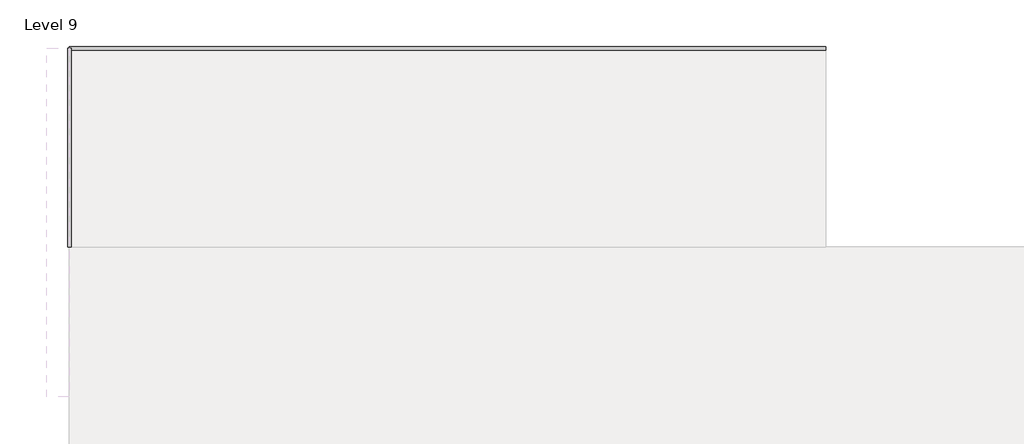
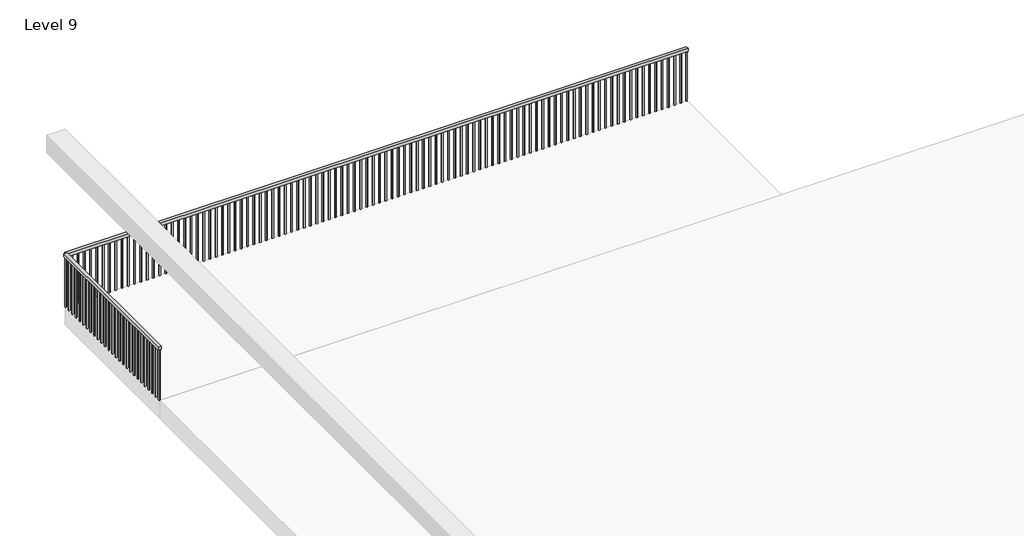
# One storey, part 3 of 5: 2 railings.
"""IFC4 building model written with IfcOpenShell, lengths in millimetres."""

from ifc_helpers import new_model, si_unit, frame, origin, place, context, project, spatial, polyline, outline, extrude, element, save

model = new_model("IFC4")

# Units and contexts
model_context = context("Model", 3, world=origin())
ifc_project = project(units=[si_unit("LENGTHUNIT", "METRE", prefix="MILLI")], contexts=[model_context])

# Site, building, storey
site = spatial("IfcSite", under=ifc_project)
building = spatial("IfcBuilding", under=site)
storey = spatial("IfcBuildingStorey", under=building, Name="Level 9", Elevation=9448.8)

# Railings
placement = place(None, origin())
element("IfcRailing", 1, ObjectType="Handrail - Rectangular", at=placement, inside=storey, context=model_context, shape_type="SweptSolid", body=[
    extrude(outline(polyline([(-13833.4638778, 17384.8237525), (-13833.4638778, 17435.6237525), (-3775.0638778, 17435.6237525), (-3775.0638778, 17384.8237525), (-13833.4638778, 17384.8237525)])), frame((0.0, 0.0, 10312.4), z_axis=(0.0, 0.0, 1.0), x_axis=(1.0, 0.0, 0.0)), (0.0, 0.0, 1.0), 50.8),
    extrude(outline(polyline([(-3886.1888778, 17400.6987525), (-3886.1888778, 17419.7487525), (-3867.1388778, 17419.7487525), (-3867.1388778, 17400.6987525), (-3886.1888778, 17400.6987525)])), frame((0.0, 0.0, 9448.8), z_axis=(0.0, 0.0, 1.0), x_axis=(1.0, 0.0, 0.0)), (0.0, 0.0, 1.0), 863.6),
    extrude(outline(polyline([(-3987.7888778, 17400.6987525), (-3987.7888778, 17419.7487525), (-3968.7388778, 17419.7487525), (-3968.7388778, 17400.6987525), (-3987.7888778, 17400.6987525)])), frame((0.0, 0.0, 9448.8), z_axis=(0.0, 0.0, 1.0), x_axis=(1.0, 0.0, 0.0)), (0.0, 0.0, 1.0), 863.6),
    extrude(outline(polyline([(-4089.3888778, 17400.6987525), (-4089.3888778, 17419.7487525), (-4070.3388778, 17419.7487525), (-4070.3388778, 17400.6987525), (-4089.3888778, 17400.6987525)])), frame((0.0, 0.0, 9448.8), z_axis=(0.0, 0.0, 1.0), x_axis=(1.0, 0.0, 0.0)), (0.0, 0.0, 1.0), 863.6),
    extrude(outline(polyline([(-4190.9888778, 17400.6987525), (-4190.9888778, 17419.7487525), (-4171.9388778, 17419.7487525), (-4171.9388778, 17400.6987525), (-4190.9888778, 17400.6987525)])), frame((0.0, 0.0, 9448.8), z_axis=(0.0, 0.0, 1.0), x_axis=(1.0, 0.0, 0.0)), (0.0, 0.0, 1.0), 863.6),
    extrude(outline(polyline([(-4292.5888778, 17400.6987525), (-4292.5888778, 17419.7487525), (-4273.5388778, 17419.7487525), (-4273.5388778, 17400.6987525), (-4292.5888778, 17400.6987525)])), frame((0.0, 0.0, 9448.8), z_axis=(0.0, 0.0, 1.0), x_axis=(1.0, 0.0, 0.0)), (0.0, 0.0, 1.0), 863.6),
    extrude(outline(polyline([(-4394.1888778, 17400.6987525), (-4394.1888778, 17419.7487525), (-4375.1388778, 17419.7487525), (-4375.1388778, 17400.6987525), (-4394.1888778, 17400.6987525)])), frame((0.0, 0.0, 9448.8), z_axis=(0.0, 0.0, 1.0), x_axis=(1.0, 0.0, 0.0)), (0.0, 0.0, 1.0), 863.6),
    extrude(outline(polyline([(-4495.7888778, 17400.6987525), (-4495.7888778, 17419.7487525), (-4476.7388778, 17419.7487525), (-4476.7388778, 17400.6987525), (-4495.7888778, 17400.6987525)])), frame((0.0, 0.0, 9448.8), z_axis=(0.0, 0.0, 1.0), x_axis=(1.0, 0.0, 0.0)), (0.0, 0.0, 1.0), 863.6),
    extrude(outline(polyline([(-4597.3888778, 17400.6987525), (-4597.3888778, 17419.7487525), (-4578.3388778, 17419.7487525), (-4578.3388778, 17400.6987525), (-4597.3888778, 17400.6987525)])), frame((0.0, 0.0, 9448.8), z_axis=(0.0, 0.0, 1.0), x_axis=(1.0, 0.0, 0.0)), (0.0, 0.0, 1.0), 863.6),
    extrude(outline(polyline([(-4698.9888778, 17400.6987525), (-4698.9888778, 17419.7487525), (-4679.9388778, 17419.7487525), (-4679.9388778, 17400.6987525), (-4698.9888778, 17400.6987525)])), frame((0.0, 0.0, 9448.8), z_axis=(0.0, 0.0, 1.0), x_axis=(1.0, 0.0, 0.0)), (0.0, 0.0, 1.0), 863.6),
    extrude(outline(polyline([(-4800.5888778, 17400.6987525), (-4800.5888778, 17419.7487525), (-4781.5388778, 17419.7487525), (-4781.5388778, 17400.6987525), (-4800.5888778, 17400.6987525)])), frame((0.0, 0.0, 9448.8), z_axis=(0.0, 0.0, 1.0), x_axis=(1.0, 0.0, 0.0)), (0.0, 0.0, 1.0), 863.6),
    extrude(outline(polyline([(-4902.1888778, 17400.6987525), (-4902.1888778, 17419.7487525), (-4883.1388778, 17419.7487525), (-4883.1388778, 17400.6987525), (-4902.1888778, 17400.6987525)])), frame((0.0, 0.0, 9448.8), z_axis=(0.0, 0.0, 1.0), x_axis=(1.0, 0.0, 0.0)), (0.0, 0.0, 1.0), 863.6),
    extrude(outline(polyline([(-5003.7888778, 17400.6987525), (-5003.7888778, 17419.7487525), (-4984.7388778, 17419.7487525), (-4984.7388778, 17400.6987525), (-5003.7888778, 17400.6987525)])), frame((0.0, 0.0, 9448.8), z_axis=(0.0, 0.0, 1.0), x_axis=(1.0, 0.0, 0.0)), (0.0, 0.0, 1.0), 863.6),
    extrude(outline(polyline([(-5105.3888778, 17400.6987525), (-5105.3888778, 17419.7487525), (-5086.3388778, 17419.7487525), (-5086.3388778, 17400.6987525), (-5105.3888778, 17400.6987525)])), frame((0.0, 0.0, 9448.8), z_axis=(0.0, 0.0, 1.0), x_axis=(1.0, 0.0, 0.0)), (0.0, 0.0, 1.0), 863.6),
    extrude(outline(polyline([(-5206.9888778, 17400.6987525), (-5206.9888778, 17419.7487525), (-5187.9388778, 17419.7487525), (-5187.9388778, 17400.6987525), (-5206.9888778, 17400.6987525)])), frame((0.0, 0.0, 9448.8), z_axis=(0.0, 0.0, 1.0), x_axis=(1.0, 0.0, 0.0)), (0.0, 0.0, 1.0), 863.6),
    extrude(outline(polyline([(-5308.5888778, 17400.6987525), (-5308.5888778, 17419.7487525), (-5289.5388778, 17419.7487525), (-5289.5388778, 17400.6987525), (-5308.5888778, 17400.6987525)])), frame((0.0, 0.0, 9448.8), z_axis=(0.0, 0.0, 1.0), x_axis=(1.0, 0.0, 0.0)), (0.0, 0.0, 1.0), 863.6),
    extrude(outline(polyline([(-5410.1888778, 17400.6987525), (-5410.1888778, 17419.7487525), (-5391.1388778, 17419.7487525), (-5391.1388778, 17400.6987525), (-5410.1888778, 17400.6987525)])), frame((0.0, 0.0, 9448.8), z_axis=(0.0, 0.0, 1.0), x_axis=(1.0, 0.0, 0.0)), (0.0, 0.0, 1.0), 863.6),
    extrude(outline(polyline([(-5511.7888778, 17400.6987525), (-5511.7888778, 17419.7487525), (-5492.7388778, 17419.7487525), (-5492.7388778, 17400.6987525), (-5511.7888778, 17400.6987525)])), frame((0.0, 0.0, 9448.8), z_axis=(0.0, 0.0, 1.0), x_axis=(1.0, 0.0, 0.0)), (0.0, 0.0, 1.0), 863.6),
    extrude(outline(polyline([(-5613.3888778, 17400.6987525), (-5613.3888778, 17419.7487525), (-5594.3388778, 17419.7487525), (-5594.3388778, 17400.6987525), (-5613.3888778, 17400.6987525)])), frame((0.0, 0.0, 9448.8), z_axis=(0.0, 0.0, 1.0), x_axis=(1.0, 0.0, 0.0)), (0.0, 0.0, 1.0), 863.6),
    extrude(outline(polyline([(-5714.9888778, 17400.6987525), (-5714.9888778, 17419.7487525), (-5695.9388778, 17419.7487525), (-5695.9388778, 17400.6987525), (-5714.9888778, 17400.6987525)])), frame((0.0, 0.0, 9448.8), z_axis=(0.0, 0.0, 1.0), x_axis=(1.0, 0.0, 0.0)), (0.0, 0.0, 1.0), 863.6),
    extrude(outline(polyline([(-5816.5888778, 17400.6987525), (-5816.5888778, 17419.7487525), (-5797.5388778, 17419.7487525), (-5797.5388778, 17400.6987525), (-5816.5888778, 17400.6987525)])), frame((0.0, 0.0, 9448.8), z_axis=(0.0, 0.0, 1.0), x_axis=(1.0, 0.0, 0.0)), (0.0, 0.0, 1.0), 863.6),
    extrude(outline(polyline([(-5918.1888778, 17400.6987525), (-5918.1888778, 17419.7487525), (-5899.1388778, 17419.7487525), (-5899.1388778, 17400.6987525), (-5918.1888778, 17400.6987525)])), frame((0.0, 0.0, 9448.8), z_axis=(0.0, 0.0, 1.0), x_axis=(1.0, 0.0, 0.0)), (0.0, 0.0, 1.0), 863.6),
    extrude(outline(polyline([(-6019.7888778, 17400.6987525), (-6019.7888778, 17419.7487525), (-6000.7388778, 17419.7487525), (-6000.7388778, 17400.6987525), (-6019.7888778, 17400.6987525)])), frame((0.0, 0.0, 9448.8), z_axis=(0.0, 0.0, 1.0), x_axis=(1.0, 0.0, 0.0)), (0.0, 0.0, 1.0), 863.6),
    extrude(outline(polyline([(-6121.3888778, 17400.6987525), (-6121.3888778, 17419.7487525), (-6102.3388778, 17419.7487525), (-6102.3388778, 17400.6987525), (-6121.3888778, 17400.6987525)])), frame((0.0, 0.0, 9448.8), z_axis=(0.0, 0.0, 1.0), x_axis=(1.0, 0.0, 0.0)), (0.0, 0.0, 1.0), 863.6),
    extrude(outline(polyline([(-6222.9888778, 17400.6987525), (-6222.9888778, 17419.7487525), (-6203.9388778, 17419.7487525), (-6203.9388778, 17400.6987525), (-6222.9888778, 17400.6987525)])), frame((0.0, 0.0, 9448.8), z_axis=(0.0, 0.0, 1.0), x_axis=(1.0, 0.0, 0.0)), (0.0, 0.0, 1.0), 863.6),
    extrude(outline(polyline([(-6324.5888778, 17400.6987525), (-6324.5888778, 17419.7487525), (-6305.5388778, 17419.7487525), (-6305.5388778, 17400.6987525), (-6324.5888778, 17400.6987525)])), frame((0.0, 0.0, 9448.8), z_axis=(0.0, 0.0, 1.0), x_axis=(1.0, 0.0, 0.0)), (0.0, 0.0, 1.0), 863.6),
    extrude(outline(polyline([(-6426.1888778, 17400.6987525), (-6426.1888778, 17419.7487525), (-6407.1388778, 17419.7487525), (-6407.1388778, 17400.6987525), (-6426.1888778, 17400.6987525)])), frame((0.0, 0.0, 9448.8), z_axis=(0.0, 0.0, 1.0), x_axis=(1.0, 0.0, 0.0)), (0.0, 0.0, 1.0), 863.6),
    extrude(outline(polyline([(-6527.7888778, 17400.6987525), (-6527.7888778, 17419.7487525), (-6508.7388778, 17419.7487525), (-6508.7388778, 17400.6987525), (-6527.7888778, 17400.6987525)])), frame((0.0, 0.0, 9448.8), z_axis=(0.0, 0.0, 1.0), x_axis=(1.0, 0.0, 0.0)), (0.0, 0.0, 1.0), 863.6),
    extrude(outline(polyline([(-6629.3888778, 17400.6987525), (-6629.3888778, 17419.7487525), (-6610.3388778, 17419.7487525), (-6610.3388778, 17400.6987525), (-6629.3888778, 17400.6987525)])), frame((0.0, 0.0, 9448.8), z_axis=(0.0, 0.0, 1.0), x_axis=(1.0, 0.0, 0.0)), (0.0, 0.0, 1.0), 863.6),
    extrude(outline(polyline([(-6730.9888778, 17400.6987525), (-6730.9888778, 17419.7487525), (-6711.9388778, 17419.7487525), (-6711.9388778, 17400.6987525), (-6730.9888778, 17400.6987525)])), frame((0.0, 0.0, 9448.8), z_axis=(0.0, 0.0, 1.0), x_axis=(1.0, 0.0, 0.0)), (0.0, 0.0, 1.0), 863.6),
    extrude(outline(polyline([(-6832.5888778, 17400.6987525), (-6832.5888778, 17419.7487525), (-6813.5388778, 17419.7487525), (-6813.5388778, 17400.6987525), (-6832.5888778, 17400.6987525)])), frame((0.0, 0.0, 9448.8), z_axis=(0.0, 0.0, 1.0), x_axis=(1.0, 0.0, 0.0)), (0.0, 0.0, 1.0), 863.6),
    extrude(outline(polyline([(-6934.1888778, 17400.6987525), (-6934.1888778, 17419.7487525), (-6915.1388778, 17419.7487525), (-6915.1388778, 17400.6987525), (-6934.1888778, 17400.6987525)])), frame((0.0, 0.0, 9448.8), z_axis=(0.0, 0.0, 1.0), x_axis=(1.0, 0.0, 0.0)), (0.0, 0.0, 1.0), 863.6),
    extrude(outline(polyline([(-7035.7888778, 17400.6987525), (-7035.7888778, 17419.7487525), (-7016.7388778, 17419.7487525), (-7016.7388778, 17400.6987525), (-7035.7888778, 17400.6987525)])), frame((0.0, 0.0, 9448.8), z_axis=(0.0, 0.0, 1.0), x_axis=(1.0, 0.0, 0.0)), (0.0, 0.0, 1.0), 863.6),
    extrude(outline(polyline([(-7137.3888778, 17400.6987525), (-7137.3888778, 17419.7487525), (-7118.3388778, 17419.7487525), (-7118.3388778, 17400.6987525), (-7137.3888778, 17400.6987525)])), frame((0.0, 0.0, 9448.8), z_axis=(0.0, 0.0, 1.0), x_axis=(1.0, 0.0, 0.0)), (0.0, 0.0, 1.0), 863.6),
    extrude(outline(polyline([(-7238.9888778, 17400.6987525), (-7238.9888778, 17419.7487525), (-7219.9388778, 17419.7487525), (-7219.9388778, 17400.6987525), (-7238.9888778, 17400.6987525)])), frame((0.0, 0.0, 9448.8), z_axis=(0.0, 0.0, 1.0), x_axis=(1.0, 0.0, 0.0)), (0.0, 0.0, 1.0), 863.6),
    extrude(outline(polyline([(-7340.5888778, 17400.6987525), (-7340.5888778, 17419.7487525), (-7321.5388778, 17419.7487525), (-7321.5388778, 17400.6987525), (-7340.5888778, 17400.6987525)])), frame((0.0, 0.0, 9448.8), z_axis=(0.0, 0.0, 1.0), x_axis=(1.0, 0.0, 0.0)), (0.0, 0.0, 1.0), 863.6),
    extrude(outline(polyline([(-7442.1888778, 17400.6987525), (-7442.1888778, 17419.7487525), (-7423.1388778, 17419.7487525), (-7423.1388778, 17400.6987525), (-7442.1888778, 17400.6987525)])), frame((0.0, 0.0, 9448.8), z_axis=(0.0, 0.0, 1.0), x_axis=(1.0, 0.0, 0.0)), (0.0, 0.0, 1.0), 863.6),
    extrude(outline(polyline([(-7543.7888778, 17400.6987525), (-7543.7888778, 17419.7487525), (-7524.7388778, 17419.7487525), (-7524.7388778, 17400.6987525), (-7543.7888778, 17400.6987525)])), frame((0.0, 0.0, 9448.8), z_axis=(0.0, 0.0, 1.0), x_axis=(1.0, 0.0, 0.0)), (0.0, 0.0, 1.0), 863.6),
    extrude(outline(polyline([(-7645.3888778, 17400.6987525), (-7645.3888778, 17419.7487525), (-7626.3388778, 17419.7487525), (-7626.3388778, 17400.6987525), (-7645.3888778, 17400.6987525)])), frame((0.0, 0.0, 9448.8), z_axis=(0.0, 0.0, 1.0), x_axis=(1.0, 0.0, 0.0)), (0.0, 0.0, 1.0), 863.6),
    extrude(outline(polyline([(-7746.9888778, 17400.6987525), (-7746.9888778, 17419.7487525), (-7727.9388778, 17419.7487525), (-7727.9388778, 17400.6987525), (-7746.9888778, 17400.6987525)])), frame((0.0, 0.0, 9448.8), z_axis=(0.0, 0.0, 1.0), x_axis=(1.0, 0.0, 0.0)), (0.0, 0.0, 1.0), 863.6),
    extrude(outline(polyline([(-7848.5888778, 17400.6987525), (-7848.5888778, 17419.7487525), (-7829.5388778, 17419.7487525), (-7829.5388778, 17400.6987525), (-7848.5888778, 17400.6987525)])), frame((0.0, 0.0, 9448.8), z_axis=(0.0, 0.0, 1.0), x_axis=(1.0, 0.0, 0.0)), (0.0, 0.0, 1.0), 863.6),
    extrude(outline(polyline([(-7950.1888778, 17400.6987525), (-7950.1888778, 17419.7487525), (-7931.1388778, 17419.7487525), (-7931.1388778, 17400.6987525), (-7950.1888778, 17400.6987525)])), frame((0.0, 0.0, 9448.8), z_axis=(0.0, 0.0, 1.0), x_axis=(1.0, 0.0, 0.0)), (0.0, 0.0, 1.0), 863.6),
    extrude(outline(polyline([(-8051.7888778, 17400.6987525), (-8051.7888778, 17419.7487525), (-8032.7388778, 17419.7487525), (-8032.7388778, 17400.6987525), (-8051.7888778, 17400.6987525)])), frame((0.0, 0.0, 9448.8), z_axis=(0.0, 0.0, 1.0), x_axis=(1.0, 0.0, 0.0)), (0.0, 0.0, 1.0), 863.6),
    extrude(outline(polyline([(-8153.3888778, 17400.6987525), (-8153.3888778, 17419.7487525), (-8134.3388778, 17419.7487525), (-8134.3388778, 17400.6987525), (-8153.3888778, 17400.6987525)])), frame((0.0, 0.0, 9448.8), z_axis=(0.0, 0.0, 1.0), x_axis=(1.0, 0.0, 0.0)), (0.0, 0.0, 1.0), 863.6),
    extrude(outline(polyline([(-8254.9888778, 17400.6987525), (-8254.9888778, 17419.7487525), (-8235.9388778, 17419.7487525), (-8235.9388778, 17400.6987525), (-8254.9888778, 17400.6987525)])), frame((0.0, 0.0, 9448.8), z_axis=(0.0, 0.0, 1.0), x_axis=(1.0, 0.0, 0.0)), (0.0, 0.0, 1.0), 863.6),
    extrude(outline(polyline([(-8356.5888778, 17400.6987525), (-8356.5888778, 17419.7487525), (-8337.5388778, 17419.7487525), (-8337.5388778, 17400.6987525), (-8356.5888778, 17400.6987525)])), frame((0.0, 0.0, 9448.8), z_axis=(0.0, 0.0, 1.0), x_axis=(1.0, 0.0, 0.0)), (0.0, 0.0, 1.0), 863.6),
    extrude(outline(polyline([(-8458.1888778, 17400.6987525), (-8458.1888778, 17419.7487525), (-8439.1388778, 17419.7487525), (-8439.1388778, 17400.6987525), (-8458.1888778, 17400.6987525)])), frame((0.0, 0.0, 9448.8), z_axis=(0.0, 0.0, 1.0), x_axis=(1.0, 0.0, 0.0)), (0.0, 0.0, 1.0), 863.6),
    extrude(outline(polyline([(-8559.7888778, 17400.6987525), (-8559.7888778, 17419.7487525), (-8540.7388778, 17419.7487525), (-8540.7388778, 17400.6987525), (-8559.7888778, 17400.6987525)])), frame((0.0, 0.0, 9448.8), z_axis=(0.0, 0.0, 1.0), x_axis=(1.0, 0.0, 0.0)), (0.0, 0.0, 1.0), 863.6),
    extrude(outline(polyline([(-8661.3888778, 17400.6987525), (-8661.3888778, 17419.7487525), (-8642.3388778, 17419.7487525), (-8642.3388778, 17400.6987525), (-8661.3888778, 17400.6987525)])), frame((0.0, 0.0, 9448.8), z_axis=(0.0, 0.0, 1.0), x_axis=(1.0, 0.0, 0.0)), (0.0, 0.0, 1.0), 863.6),
    extrude(outline(polyline([(-8762.9888778, 17400.6987525), (-8762.9888778, 17419.7487525), (-8743.9388778, 17419.7487525), (-8743.9388778, 17400.6987525), (-8762.9888778, 17400.6987525)])), frame((0.0, 0.0, 9448.8), z_axis=(0.0, 0.0, 1.0), x_axis=(1.0, 0.0, 0.0)), (0.0, 0.0, 1.0), 863.6),
    extrude(outline(polyline([(-8864.5888778, 17400.6987525), (-8864.5888778, 17419.7487525), (-8845.5388778, 17419.7487525), (-8845.5388778, 17400.6987525), (-8864.5888778, 17400.6987525)])), frame((0.0, 0.0, 9448.8), z_axis=(0.0, 0.0, 1.0), x_axis=(1.0, 0.0, 0.0)), (0.0, 0.0, 1.0), 863.6),
    extrude(outline(polyline([(-8966.1888778, 17400.6987525), (-8966.1888778, 17419.7487525), (-8947.1388778, 17419.7487525), (-8947.1388778, 17400.6987525), (-8966.1888778, 17400.6987525)])), frame((0.0, 0.0, 9448.8), z_axis=(0.0, 0.0, 1.0), x_axis=(1.0, 0.0, 0.0)), (0.0, 0.0, 1.0), 863.6),
    extrude(outline(polyline([(-9067.7888778, 17400.6987525), (-9067.7888778, 17419.7487525), (-9048.7388778, 17419.7487525), (-9048.7388778, 17400.6987525), (-9067.7888778, 17400.6987525)])), frame((0.0, 0.0, 9448.8), z_axis=(0.0, 0.0, 1.0), x_axis=(1.0, 0.0, 0.0)), (0.0, 0.0, 1.0), 863.6),
    extrude(outline(polyline([(-9169.3888778, 17400.6987525), (-9169.3888778, 17419.7487525), (-9150.3388778, 17419.7487525), (-9150.3388778, 17400.6987525), (-9169.3888778, 17400.6987525)])), frame((0.0, 0.0, 9448.8), z_axis=(0.0, 0.0, 1.0), x_axis=(1.0, 0.0, 0.0)), (0.0, 0.0, 1.0), 863.6),
    extrude(outline(polyline([(-9270.9888778, 17400.6987525), (-9270.9888778, 17419.7487525), (-9251.9388778, 17419.7487525), (-9251.9388778, 17400.6987525), (-9270.9888778, 17400.6987525)])), frame((0.0, 0.0, 9448.8), z_axis=(0.0, 0.0, 1.0), x_axis=(1.0, 0.0, 0.0)), (0.0, 0.0, 1.0), 863.6),
    extrude(outline(polyline([(-9372.5888778, 17400.6987525), (-9372.5888778, 17419.7487525), (-9353.5388778, 17419.7487525), (-9353.5388778, 17400.6987525), (-9372.5888778, 17400.6987525)])), frame((0.0, 0.0, 9448.8), z_axis=(0.0, 0.0, 1.0), x_axis=(1.0, 0.0, 0.0)), (0.0, 0.0, 1.0), 863.6),
    extrude(outline(polyline([(-9474.1888778, 17400.6987525), (-9474.1888778, 17419.7487525), (-9455.1388778, 17419.7487525), (-9455.1388778, 17400.6987525), (-9474.1888778, 17400.6987525)])), frame((0.0, 0.0, 9448.8), z_axis=(0.0, 0.0, 1.0), x_axis=(1.0, 0.0, 0.0)), (0.0, 0.0, 1.0), 863.6),
    extrude(outline(polyline([(-9575.7888778, 17400.6987525), (-9575.7888778, 17419.7487525), (-9556.7388778, 17419.7487525), (-9556.7388778, 17400.6987525), (-9575.7888778, 17400.6987525)])), frame((0.0, 0.0, 9448.8), z_axis=(0.0, 0.0, 1.0), x_axis=(1.0, 0.0, 0.0)), (0.0, 0.0, 1.0), 863.6),
    extrude(outline(polyline([(-9677.3888778, 17400.6987525), (-9677.3888778, 17419.7487525), (-9658.3388778, 17419.7487525), (-9658.3388778, 17400.6987525), (-9677.3888778, 17400.6987525)])), frame((0.0, 0.0, 9448.8), z_axis=(0.0, 0.0, 1.0), x_axis=(1.0, 0.0, 0.0)), (0.0, 0.0, 1.0), 863.6),
    extrude(outline(polyline([(-9778.9888778, 17400.6987525), (-9778.9888778, 17419.7487525), (-9759.9388778, 17419.7487525), (-9759.9388778, 17400.6987525), (-9778.9888778, 17400.6987525)])), frame((0.0, 0.0, 9448.8), z_axis=(0.0, 0.0, 1.0), x_axis=(1.0, 0.0, 0.0)), (0.0, 0.0, 1.0), 863.6),
    extrude(outline(polyline([(-9880.5888778, 17400.6987525), (-9880.5888778, 17419.7487525), (-9861.5388778, 17419.7487525), (-9861.5388778, 17400.6987525), (-9880.5888778, 17400.6987525)])), frame((0.0, 0.0, 9448.8), z_axis=(0.0, 0.0, 1.0), x_axis=(1.0, 0.0, 0.0)), (0.0, 0.0, 1.0), 863.6),
    extrude(outline(polyline([(-9982.1888778, 17400.6987525), (-9982.1888778, 17419.7487525), (-9963.1388778, 17419.7487525), (-9963.1388778, 17400.6987525), (-9982.1888778, 17400.6987525)])), frame((0.0, 0.0, 9448.8), z_axis=(0.0, 0.0, 1.0), x_axis=(1.0, 0.0, 0.0)), (0.0, 0.0, 1.0), 863.6),
    extrude(outline(polyline([(-10083.7888778, 17400.6987525), (-10083.7888778, 17419.7487525), (-10064.7388778, 17419.7487525), (-10064.7388778, 17400.6987525), (-10083.7888778, 17400.6987525)])), frame((0.0, 0.0, 9448.8), z_axis=(0.0, 0.0, 1.0), x_axis=(1.0, 0.0, 0.0)), (0.0, 0.0, 1.0), 863.6),
    extrude(outline(polyline([(-10185.3888778, 17400.6987525), (-10185.3888778, 17419.7487525), (-10166.3388778, 17419.7487525), (-10166.3388778, 17400.6987525), (-10185.3888778, 17400.6987525)])), frame((0.0, 0.0, 9448.8), z_axis=(0.0, 0.0, 1.0), x_axis=(1.0, 0.0, 0.0)), (0.0, 0.0, 1.0), 863.6),
    extrude(outline(polyline([(-10286.9888778, 17400.6987525), (-10286.9888778, 17419.7487525), (-10267.9388778, 17419.7487525), (-10267.9388778, 17400.6987525), (-10286.9888778, 17400.6987525)])), frame((0.0, 0.0, 9448.8), z_axis=(0.0, 0.0, 1.0), x_axis=(1.0, 0.0, 0.0)), (0.0, 0.0, 1.0), 863.6),
    extrude(outline(polyline([(-10388.5888778, 17400.6987525), (-10388.5888778, 17419.7487525), (-10369.5388778, 17419.7487525), (-10369.5388778, 17400.6987525), (-10388.5888778, 17400.6987525)])), frame((0.0, 0.0, 9448.8), z_axis=(0.0, 0.0, 1.0), x_axis=(1.0, 0.0, 0.0)), (0.0, 0.0, 1.0), 863.6),
    extrude(outline(polyline([(-10490.1888778, 17400.6987525), (-10490.1888778, 17419.7487525), (-10471.1388778, 17419.7487525), (-10471.1388778, 17400.6987525), (-10490.1888778, 17400.6987525)])), frame((0.0, 0.0, 9448.8), z_axis=(0.0, 0.0, 1.0), x_axis=(1.0, 0.0, 0.0)), (0.0, 0.0, 1.0), 863.6),
    extrude(outline(polyline([(-10591.7888778, 17400.6987525), (-10591.7888778, 17419.7487525), (-10572.7388778, 17419.7487525), (-10572.7388778, 17400.6987525), (-10591.7888778, 17400.6987525)])), frame((0.0, 0.0, 9448.8), z_axis=(0.0, 0.0, 1.0), x_axis=(1.0, 0.0, 0.0)), (0.0, 0.0, 1.0), 863.6),
    extrude(outline(polyline([(-10693.3888778, 17400.6987525), (-10693.3888778, 17419.7487525), (-10674.3388778, 17419.7487525), (-10674.3388778, 17400.6987525), (-10693.3888778, 17400.6987525)])), frame((0.0, 0.0, 9448.8), z_axis=(0.0, 0.0, 1.0), x_axis=(1.0, 0.0, 0.0)), (0.0, 0.0, 1.0), 863.6),
    extrude(outline(polyline([(-10794.9888778, 17400.6987525), (-10794.9888778, 17419.7487525), (-10775.9388778, 17419.7487525), (-10775.9388778, 17400.6987525), (-10794.9888778, 17400.6987525)])), frame((0.0, 0.0, 9448.8), z_axis=(0.0, 0.0, 1.0), x_axis=(1.0, 0.0, 0.0)), (0.0, 0.0, 1.0), 863.6),
    extrude(outline(polyline([(-10896.5888778, 17400.6987525), (-10896.5888778, 17419.7487525), (-10877.5388778, 17419.7487525), (-10877.5388778, 17400.6987525), (-10896.5888778, 17400.6987525)])), frame((0.0, 0.0, 9448.8), z_axis=(0.0, 0.0, 1.0), x_axis=(1.0, 0.0, 0.0)), (0.0, 0.0, 1.0), 863.6),
    extrude(outline(polyline([(-10998.1888778, 17400.6987525), (-10998.1888778, 17419.7487525), (-10979.1388778, 17419.7487525), (-10979.1388778, 17400.6987525), (-10998.1888778, 17400.6987525)])), frame((0.0, 0.0, 9448.8), z_axis=(0.0, 0.0, 1.0), x_axis=(1.0, 0.0, 0.0)), (0.0, 0.0, 1.0), 863.6),
    extrude(outline(polyline([(-11099.7888778, 17400.6987525), (-11099.7888778, 17419.7487525), (-11080.7388778, 17419.7487525), (-11080.7388778, 17400.6987525), (-11099.7888778, 17400.6987525)])), frame((0.0, 0.0, 9448.8), z_axis=(0.0, 0.0, 1.0), x_axis=(1.0, 0.0, 0.0)), (0.0, 0.0, 1.0), 863.6),
    extrude(outline(polyline([(-11201.3888778, 17400.6987525), (-11201.3888778, 17419.7487525), (-11182.3388778, 17419.7487525), (-11182.3388778, 17400.6987525), (-11201.3888778, 17400.6987525)])), frame((0.0, 0.0, 9448.8), z_axis=(0.0, 0.0, 1.0), x_axis=(1.0, 0.0, 0.0)), (0.0, 0.0, 1.0), 863.6),
    extrude(outline(polyline([(-11302.9888778, 17400.6987525), (-11302.9888778, 17419.7487525), (-11283.9388778, 17419.7487525), (-11283.9388778, 17400.6987525), (-11302.9888778, 17400.6987525)])), frame((0.0, 0.0, 9448.8), z_axis=(0.0, 0.0, 1.0), x_axis=(1.0, 0.0, 0.0)), (0.0, 0.0, 1.0), 863.6),
    extrude(outline(polyline([(-11404.5888778, 17400.6987525), (-11404.5888778, 17419.7487525), (-11385.5388778, 17419.7487525), (-11385.5388778, 17400.6987525), (-11404.5888778, 17400.6987525)])), frame((0.0, 0.0, 9448.8), z_axis=(0.0, 0.0, 1.0), x_axis=(1.0, 0.0, 0.0)), (0.0, 0.0, 1.0), 863.6),
    extrude(outline(polyline([(-11506.1888778, 17400.6987525), (-11506.1888778, 17419.7487525), (-11487.1388778, 17419.7487525), (-11487.1388778, 17400.6987525), (-11506.1888778, 17400.6987525)])), frame((0.0, 0.0, 9448.8), z_axis=(0.0, 0.0, 1.0), x_axis=(1.0, 0.0, 0.0)), (0.0, 0.0, 1.0), 863.6),
    extrude(outline(polyline([(-11607.7888778, 17400.6987525), (-11607.7888778, 17419.7487525), (-11588.7388778, 17419.7487525), (-11588.7388778, 17400.6987525), (-11607.7888778, 17400.6987525)])), frame((0.0, 0.0, 9448.8), z_axis=(0.0, 0.0, 1.0), x_axis=(1.0, 0.0, 0.0)), (0.0, 0.0, 1.0), 863.6),
    extrude(outline(polyline([(-11709.3888778, 17400.6987525), (-11709.3888778, 17419.7487525), (-11690.3388778, 17419.7487525), (-11690.3388778, 17400.6987525), (-11709.3888778, 17400.6987525)])), frame((0.0, 0.0, 9448.8), z_axis=(0.0, 0.0, 1.0), x_axis=(1.0, 0.0, 0.0)), (0.0, 0.0, 1.0), 863.6),
    extrude(outline(polyline([(-11810.9888778, 17400.6987525), (-11810.9888778, 17419.7487525), (-11791.9388778, 17419.7487525), (-11791.9388778, 17400.6987525), (-11810.9888778, 17400.6987525)])), frame((0.0, 0.0, 9448.8), z_axis=(0.0, 0.0, 1.0), x_axis=(1.0, 0.0, 0.0)), (0.0, 0.0, 1.0), 863.6),
    extrude(outline(polyline([(-11912.5888778, 17400.6987525), (-11912.5888778, 17419.7487525), (-11893.5388778, 17419.7487525), (-11893.5388778, 17400.6987525), (-11912.5888778, 17400.6987525)])), frame((0.0, 0.0, 9448.8), z_axis=(0.0, 0.0, 1.0), x_axis=(1.0, 0.0, 0.0)), (0.0, 0.0, 1.0), 863.6),
    extrude(outline(polyline([(-12014.1888778, 17400.6987525), (-12014.1888778, 17419.7487525), (-11995.1388778, 17419.7487525), (-11995.1388778, 17400.6987525), (-12014.1888778, 17400.6987525)])), frame((0.0, 0.0, 9448.8), z_axis=(0.0, 0.0, 1.0), x_axis=(1.0, 0.0, 0.0)), (0.0, 0.0, 1.0), 863.6),
    extrude(outline(polyline([(-12115.7888778, 17400.6987525), (-12115.7888778, 17419.7487525), (-12096.7388778, 17419.7487525), (-12096.7388778, 17400.6987525), (-12115.7888778, 17400.6987525)])), frame((0.0, 0.0, 9448.8), z_axis=(0.0, 0.0, 1.0), x_axis=(1.0, 0.0, 0.0)), (0.0, 0.0, 1.0), 863.6),
    extrude(outline(polyline([(-12217.3888778, 17400.6987525), (-12217.3888778, 17419.7487525), (-12198.3388778, 17419.7487525), (-12198.3388778, 17400.6987525), (-12217.3888778, 17400.6987525)])), frame((0.0, 0.0, 9448.8), z_axis=(0.0, 0.0, 1.0), x_axis=(1.0, 0.0, 0.0)), (0.0, 0.0, 1.0), 863.6),
    extrude(outline(polyline([(-12318.9888778, 17400.6987525), (-12318.9888778, 17419.7487525), (-12299.9388778, 17419.7487525), (-12299.9388778, 17400.6987525), (-12318.9888778, 17400.6987525)])), frame((0.0, 0.0, 9448.8), z_axis=(0.0, 0.0, 1.0), x_axis=(1.0, 0.0, 0.0)), (0.0, 0.0, 1.0), 863.6),
    extrude(outline(polyline([(-12420.5888778, 17400.6987525), (-12420.5888778, 17419.7487525), (-12401.5388778, 17419.7487525), (-12401.5388778, 17400.6987525), (-12420.5888778, 17400.6987525)])), frame((0.0, 0.0, 9448.8), z_axis=(0.0, 0.0, 1.0), x_axis=(1.0, 0.0, 0.0)), (0.0, 0.0, 1.0), 863.6),
    extrude(outline(polyline([(-12522.1888778, 17400.6987525), (-12522.1888778, 17419.7487525), (-12503.1388778, 17419.7487525), (-12503.1388778, 17400.6987525), (-12522.1888778, 17400.6987525)])), frame((0.0, 0.0, 9448.8), z_axis=(0.0, 0.0, 1.0), x_axis=(1.0, 0.0, 0.0)), (0.0, 0.0, 1.0), 863.6),
    extrude(outline(polyline([(-12623.7888778, 17400.6987525), (-12623.7888778, 17419.7487525), (-12604.7388778, 17419.7487525), (-12604.7388778, 17400.6987525), (-12623.7888778, 17400.6987525)])), frame((0.0, 0.0, 9448.8), z_axis=(0.0, 0.0, 1.0), x_axis=(1.0, 0.0, 0.0)), (0.0, 0.0, 1.0), 863.6),
    extrude(outline(polyline([(-12725.3888778, 17400.6987525), (-12725.3888778, 17419.7487525), (-12706.3388778, 17419.7487525), (-12706.3388778, 17400.6987525), (-12725.3888778, 17400.6987525)])), frame((0.0, 0.0, 9448.8), z_axis=(0.0, 0.0, 1.0), x_axis=(1.0, 0.0, 0.0)), (0.0, 0.0, 1.0), 863.6),
    extrude(outline(polyline([(-12826.9888778, 17400.6987525), (-12826.9888778, 17419.7487525), (-12807.9388778, 17419.7487525), (-12807.9388778, 17400.6987525), (-12826.9888778, 17400.6987525)])), frame((0.0, 0.0, 9448.8), z_axis=(0.0, 0.0, 1.0), x_axis=(1.0, 0.0, 0.0)), (0.0, 0.0, 1.0), 863.6),
    extrude(outline(polyline([(-12928.5888778, 17400.6987525), (-12928.5888778, 17419.7487525), (-12909.5388778, 17419.7487525), (-12909.5388778, 17400.6987525), (-12928.5888778, 17400.6987525)])), frame((0.0, 0.0, 9448.8), z_axis=(0.0, 0.0, 1.0), x_axis=(1.0, 0.0, 0.0)), (0.0, 0.0, 1.0), 863.6),
    extrude(outline(polyline([(-13030.1888778, 17400.6987525), (-13030.1888778, 17419.7487525), (-13011.1388778, 17419.7487525), (-13011.1388778, 17400.6987525), (-13030.1888778, 17400.6987525)])), frame((0.0, 0.0, 9448.8), z_axis=(0.0, 0.0, 1.0), x_axis=(1.0, 0.0, 0.0)), (0.0, 0.0, 1.0), 863.6),
    extrude(outline(polyline([(-13131.7888778, 17400.6987525), (-13131.7888778, 17419.7487525), (-13112.7388778, 17419.7487525), (-13112.7388778, 17400.6987525), (-13131.7888778, 17400.6987525)])), frame((0.0, 0.0, 9448.8), z_axis=(0.0, 0.0, 1.0), x_axis=(1.0, 0.0, 0.0)), (0.0, 0.0, 1.0), 863.6),
    extrude(outline(polyline([(-13233.3888778, 17400.6987525), (-13233.3888778, 17419.7487525), (-13214.3388778, 17419.7487525), (-13214.3388778, 17400.6987525), (-13233.3888778, 17400.6987525)])), frame((0.0, 0.0, 9448.8), z_axis=(0.0, 0.0, 1.0), x_axis=(1.0, 0.0, 0.0)), (0.0, 0.0, 1.0), 863.6),
    extrude(outline(polyline([(-13334.9888778, 17400.6987525), (-13334.9888778, 17419.7487525), (-13315.9388778, 17419.7487525), (-13315.9388778, 17400.6987525), (-13334.9888778, 17400.6987525)])), frame((0.0, 0.0, 9448.8), z_axis=(0.0, 0.0, 1.0), x_axis=(1.0, 0.0, 0.0)), (0.0, 0.0, 1.0), 863.6),
    extrude(outline(polyline([(-13436.5888778, 17400.6987525), (-13436.5888778, 17419.7487525), (-13417.5388778, 17419.7487525), (-13417.5388778, 17400.6987525), (-13436.5888778, 17400.6987525)])), frame((0.0, 0.0, 9448.8), z_axis=(0.0, 0.0, 1.0), x_axis=(1.0, 0.0, 0.0)), (0.0, 0.0, 1.0), 863.6),
    extrude(outline(polyline([(-13538.1888778, 17400.6987525), (-13538.1888778, 17419.7487525), (-13519.1388778, 17419.7487525), (-13519.1388778, 17400.6987525), (-13538.1888778, 17400.6987525)])), frame((0.0, 0.0, 9448.8), z_axis=(0.0, 0.0, 1.0), x_axis=(1.0, 0.0, 0.0)), (0.0, 0.0, 1.0), 863.6),
    extrude(outline(polyline([(-13639.7888778, 17400.6987525), (-13639.7888778, 17419.7487525), (-13620.7388778, 17419.7487525), (-13620.7388778, 17400.6987525), (-13639.7888778, 17400.6987525)])), frame((0.0, 0.0, 9448.8), z_axis=(0.0, 0.0, 1.0), x_axis=(1.0, 0.0, 0.0)), (0.0, 0.0, 1.0), 863.6),
    extrude(outline(polyline([(-13741.3888778, 17400.6987525), (-13741.3888778, 17419.7487525), (-13722.3388778, 17419.7487525), (-13722.3388778, 17400.6987525), (-13741.3888778, 17400.6987525)])), frame((0.0, 0.0, 9448.8), z_axis=(0.0, 0.0, 1.0), x_axis=(1.0, 0.0, 0.0)), (0.0, 0.0, 1.0), 863.6),
    extrude(outline(polyline([(-3794.1138778, 17400.6987525), (-3794.1138778, 17419.7487525), (-3775.0638778, 17419.7487525), (-3775.0638778, 17400.6987525), (-3794.1138778, 17400.6987525)])), frame((0.0, 0.0, 9448.8), z_axis=(0.0, 0.0, 1.0), x_axis=(1.0, 0.0, 0.0)), (0.0, 0.0, 1.0), 863.6),
    extrude(outline(polyline([(-13833.4638778, 17400.6987525), (-13833.4638778, 17419.7487525), (-13814.4138778, 17419.7487525), (-13814.4138778, 17400.6987525), (-13833.4638778, 17400.6987525)])), frame((0.0, 0.0, 9448.8), z_axis=(0.0, 0.0, 1.0), x_axis=(1.0, 0.0, 0.0)), (0.0, 0.0, 1.0), 863.6),
])
element("IfcRailing", 2, ObjectType="Handrail - Rectangular", at=placement, inside=storey, context=model_context, shape_type="SweptSolid", body=[
    extrude(outline(polyline([(-13808.0638778, 14768.6237525), (-13858.8638778, 14768.6237525), (-13858.8638778, 17410.2237525), (-13808.0638778, 17410.2237525), (-13808.0638778, 14768.6237525)])), frame((0.0, 0.0, 10312.4), z_axis=(0.0, 0.0, 1.0), x_axis=(1.0, 0.0, 0.0)), (0.0, 0.0, 1.0), 50.8),
    extrude(outline(polyline([(-13823.9388778, 17299.0987525), (-13842.9888778, 17299.0987525), (-13842.9888778, 17318.1487525), (-13823.9388778, 17318.1487525), (-13823.9388778, 17299.0987525)])), frame((0.0, 0.0, 9448.8), z_axis=(0.0, 0.0, 1.0), x_axis=(1.0, 0.0, 0.0)), (0.0, 0.0, 1.0), 863.6),
    extrude(outline(polyline([(-13823.9388778, 17197.4987525), (-13842.9888778, 17197.4987525), (-13842.9888778, 17216.5487525), (-13823.9388778, 17216.5487525), (-13823.9388778, 17197.4987525)])), frame((0.0, 0.0, 9448.8), z_axis=(0.0, 0.0, 1.0), x_axis=(1.0, 0.0, 0.0)), (0.0, 0.0, 1.0), 863.6),
    extrude(outline(polyline([(-13823.9388778, 17095.8987525), (-13842.9888778, 17095.8987525), (-13842.9888778, 17114.9487525), (-13823.9388778, 17114.9487525), (-13823.9388778, 17095.8987525)])), frame((0.0, 0.0, 9448.8), z_axis=(0.0, 0.0, 1.0), x_axis=(1.0, 0.0, 0.0)), (0.0, 0.0, 1.0), 863.6),
    extrude(outline(polyline([(-13823.9388778, 16994.2987525), (-13842.9888778, 16994.2987525), (-13842.9888778, 17013.3487525), (-13823.9388778, 17013.3487525), (-13823.9388778, 16994.2987525)])), frame((0.0, 0.0, 9448.8), z_axis=(0.0, 0.0, 1.0), x_axis=(1.0, 0.0, 0.0)), (0.0, 0.0, 1.0), 863.6),
    extrude(outline(polyline([(-13823.9388778, 16892.6987525), (-13842.9888778, 16892.6987525), (-13842.9888778, 16911.7487525), (-13823.9388778, 16911.7487525), (-13823.9388778, 16892.6987525)])), frame((0.0, 0.0, 9448.8), z_axis=(0.0, 0.0, 1.0), x_axis=(1.0, 0.0, 0.0)), (0.0, 0.0, 1.0), 863.6),
    extrude(outline(polyline([(-13823.9388778, 16791.0987525), (-13842.9888778, 16791.0987525), (-13842.9888778, 16810.1487525), (-13823.9388778, 16810.1487525), (-13823.9388778, 16791.0987525)])), frame((0.0, 0.0, 9448.8), z_axis=(0.0, 0.0, 1.0), x_axis=(1.0, 0.0, 0.0)), (0.0, 0.0, 1.0), 863.6),
    extrude(outline(polyline([(-13823.9388778, 16689.4987525), (-13842.9888778, 16689.4987525), (-13842.9888778, 16708.5487525), (-13823.9388778, 16708.5487525), (-13823.9388778, 16689.4987525)])), frame((0.0, 0.0, 9448.8), z_axis=(0.0, 0.0, 1.0), x_axis=(1.0, 0.0, 0.0)), (0.0, 0.0, 1.0), 863.6),
    extrude(outline(polyline([(-13823.9388778, 16587.8987525), (-13842.9888778, 16587.8987525), (-13842.9888778, 16606.9487525), (-13823.9388778, 16606.9487525), (-13823.9388778, 16587.8987525)])), frame((0.0, 0.0, 9448.8), z_axis=(0.0, 0.0, 1.0), x_axis=(1.0, 0.0, 0.0)), (0.0, 0.0, 1.0), 863.6),
    extrude(outline(polyline([(-13823.9388778, 16486.2987525), (-13842.9888778, 16486.2987525), (-13842.9888778, 16505.3487525), (-13823.9388778, 16505.3487525), (-13823.9388778, 16486.2987525)])), frame((0.0, 0.0, 9448.8), z_axis=(0.0, 0.0, 1.0), x_axis=(1.0, 0.0, 0.0)), (0.0, 0.0, 1.0), 863.6),
    extrude(outline(polyline([(-13823.9388778, 16384.6987525), (-13842.9888778, 16384.6987525), (-13842.9888778, 16403.7487525), (-13823.9388778, 16403.7487525), (-13823.9388778, 16384.6987525)])), frame((0.0, 0.0, 9448.8), z_axis=(0.0, 0.0, 1.0), x_axis=(1.0, 0.0, 0.0)), (0.0, 0.0, 1.0), 863.6),
    extrude(outline(polyline([(-13823.9388778, 16283.0987525), (-13842.9888778, 16283.0987525), (-13842.9888778, 16302.1487525), (-13823.9388778, 16302.1487525), (-13823.9388778, 16283.0987525)])), frame((0.0, 0.0, 9448.8), z_axis=(0.0, 0.0, 1.0), x_axis=(1.0, 0.0, 0.0)), (0.0, 0.0, 1.0), 863.6),
    extrude(outline(polyline([(-13823.9388778, 16181.4987525), (-13842.9888778, 16181.4987525), (-13842.9888778, 16200.5487525), (-13823.9388778, 16200.5487525), (-13823.9388778, 16181.4987525)])), frame((0.0, 0.0, 9448.8), z_axis=(0.0, 0.0, 1.0), x_axis=(1.0, 0.0, 0.0)), (0.0, 0.0, 1.0), 863.6),
    extrude(outline(polyline([(-13823.9388778, 16079.8987525), (-13842.9888778, 16079.8987525), (-13842.9888778, 16098.9487525), (-13823.9388778, 16098.9487525), (-13823.9388778, 16079.8987525)])), frame((0.0, 0.0, 9448.8), z_axis=(0.0, 0.0, 1.0), x_axis=(1.0, 0.0, 0.0)), (0.0, 0.0, 1.0), 863.6),
    extrude(outline(polyline([(-13823.9388778, 15978.2987525), (-13842.9888778, 15978.2987525), (-13842.9888778, 15997.3487525), (-13823.9388778, 15997.3487525), (-13823.9388778, 15978.2987525)])), frame((0.0, 0.0, 9448.8), z_axis=(0.0, 0.0, 1.0), x_axis=(1.0, 0.0, 0.0)), (0.0, 0.0, 1.0), 863.6),
    extrude(outline(polyline([(-13823.9388778, 15876.6987525), (-13842.9888778, 15876.6987525), (-13842.9888778, 15895.7487525), (-13823.9388778, 15895.7487525), (-13823.9388778, 15876.6987525)])), frame((0.0, 0.0, 9448.8), z_axis=(0.0, 0.0, 1.0), x_axis=(1.0, 0.0, 0.0)), (0.0, 0.0, 1.0), 863.6),
    extrude(outline(polyline([(-13823.9388778, 15775.0987525), (-13842.9888778, 15775.0987525), (-13842.9888778, 15794.1487525), (-13823.9388778, 15794.1487525), (-13823.9388778, 15775.0987525)])), frame((0.0, 0.0, 9448.8), z_axis=(0.0, 0.0, 1.0), x_axis=(1.0, 0.0, 0.0)), (0.0, 0.0, 1.0), 863.6),
    extrude(outline(polyline([(-13823.9388778, 15673.4987525), (-13842.9888778, 15673.4987525), (-13842.9888778, 15692.5487525), (-13823.9388778, 15692.5487525), (-13823.9388778, 15673.4987525)])), frame((0.0, 0.0, 9448.8), z_axis=(0.0, 0.0, 1.0), x_axis=(1.0, 0.0, 0.0)), (0.0, 0.0, 1.0), 863.6),
    extrude(outline(polyline([(-13823.9388778, 15571.8987525), (-13842.9888778, 15571.8987525), (-13842.9888778, 15590.9487525), (-13823.9388778, 15590.9487525), (-13823.9388778, 15571.8987525)])), frame((0.0, 0.0, 9448.8), z_axis=(0.0, 0.0, 1.0), x_axis=(1.0, 0.0, 0.0)), (0.0, 0.0, 1.0), 863.6),
    extrude(outline(polyline([(-13823.9388778, 15470.2987525), (-13842.9888778, 15470.2987525), (-13842.9888778, 15489.3487525), (-13823.9388778, 15489.3487525), (-13823.9388778, 15470.2987525)])), frame((0.0, 0.0, 9448.8), z_axis=(0.0, 0.0, 1.0), x_axis=(1.0, 0.0, 0.0)), (0.0, 0.0, 1.0), 863.6),
    extrude(outline(polyline([(-13823.9388778, 15368.6987525), (-13842.9888778, 15368.6987525), (-13842.9888778, 15387.7487525), (-13823.9388778, 15387.7487525), (-13823.9388778, 15368.6987525)])), frame((0.0, 0.0, 9448.8), z_axis=(0.0, 0.0, 1.0), x_axis=(1.0, 0.0, 0.0)), (0.0, 0.0, 1.0), 863.6),
    extrude(outline(polyline([(-13823.9388778, 15267.0987525), (-13842.9888778, 15267.0987525), (-13842.9888778, 15286.1487525), (-13823.9388778, 15286.1487525), (-13823.9388778, 15267.0987525)])), frame((0.0, 0.0, 9448.8), z_axis=(0.0, 0.0, 1.0), x_axis=(1.0, 0.0, 0.0)), (0.0, 0.0, 1.0), 863.6),
    extrude(outline(polyline([(-13823.9388778, 15165.4987525), (-13842.9888778, 15165.4987525), (-13842.9888778, 15184.5487525), (-13823.9388778, 15184.5487525), (-13823.9388778, 15165.4987525)])), frame((0.0, 0.0, 9448.8), z_axis=(0.0, 0.0, 1.0), x_axis=(1.0, 0.0, 0.0)), (0.0, 0.0, 1.0), 863.6),
    extrude(outline(polyline([(-13823.9388778, 15063.8987525), (-13842.9888778, 15063.8987525), (-13842.9888778, 15082.9487525), (-13823.9388778, 15082.9487525), (-13823.9388778, 15063.8987525)])), frame((0.0, 0.0, 9448.8), z_axis=(0.0, 0.0, 1.0), x_axis=(1.0, 0.0, 0.0)), (0.0, 0.0, 1.0), 863.6),
    extrude(outline(polyline([(-13823.9388778, 14962.2987525), (-13842.9888778, 14962.2987525), (-13842.9888778, 14981.3487525), (-13823.9388778, 14981.3487525), (-13823.9388778, 14962.2987525)])), frame((0.0, 0.0, 9448.8), z_axis=(0.0, 0.0, 1.0), x_axis=(1.0, 0.0, 0.0)), (0.0, 0.0, 1.0), 863.6),
    extrude(outline(polyline([(-13823.9388778, 14860.6987525), (-13842.9888778, 14860.6987525), (-13842.9888778, 14879.7487525), (-13823.9388778, 14879.7487525), (-13823.9388778, 14860.6987525)])), frame((0.0, 0.0, 9448.8), z_axis=(0.0, 0.0, 1.0), x_axis=(1.0, 0.0, 0.0)), (0.0, 0.0, 1.0), 863.6),
    extrude(outline(polyline([(-13823.9388778, 17391.1737525), (-13842.9888778, 17391.1737525), (-13842.9888778, 17410.2237525), (-13823.9388778, 17410.2237525), (-13823.9388778, 17391.1737525)])), frame((0.0, 0.0, 9448.8), z_axis=(0.0, 0.0, 1.0), x_axis=(1.0, 0.0, 0.0)), (0.0, 0.0, 1.0), 863.6),
    extrude(outline(polyline([(-13823.9388778, 14768.6237525), (-13842.9888778, 14768.6237525), (-13842.9888778, 14787.6737525), (-13823.9388778, 14787.6737525), (-13823.9388778, 14768.6237525)])), frame((0.0, 0.0, 9448.8), z_axis=(0.0, 0.0, 1.0), x_axis=(1.0, 0.0, 0.0)), (0.0, 0.0, 1.0), 863.6),
])

save(model, "model.ifc")

# Revit data of these elements
# Type "Handrail - Rectangular"
#   Assembly Code = "C2010400"
#   built-in parameter 1008612 = 0.0416667 (stored number, unit not read)
#   built-in parameter 1008611 = 0.0416667 (stored number, unit not read)
#   built-in parameter 1008609 = 0.333333 (stored number, unit not read)
#   built-in parameter 1008604 = 0.166667 (stored number, unit not read)
#   built-in parameter 1008603 = 0.166667 (stored number, unit not read)
#   Railing Height = 3' - 0"
#   built-in parameter 1008630 = 2
#   built-in parameter 1008610 = 2
#   built-in parameter 1008618 = Baluster - Square : 3/4"
# Elements 1, 2 (IfcRailing, "Handrail - Rectangular")
#   Phase Created = New Construction
